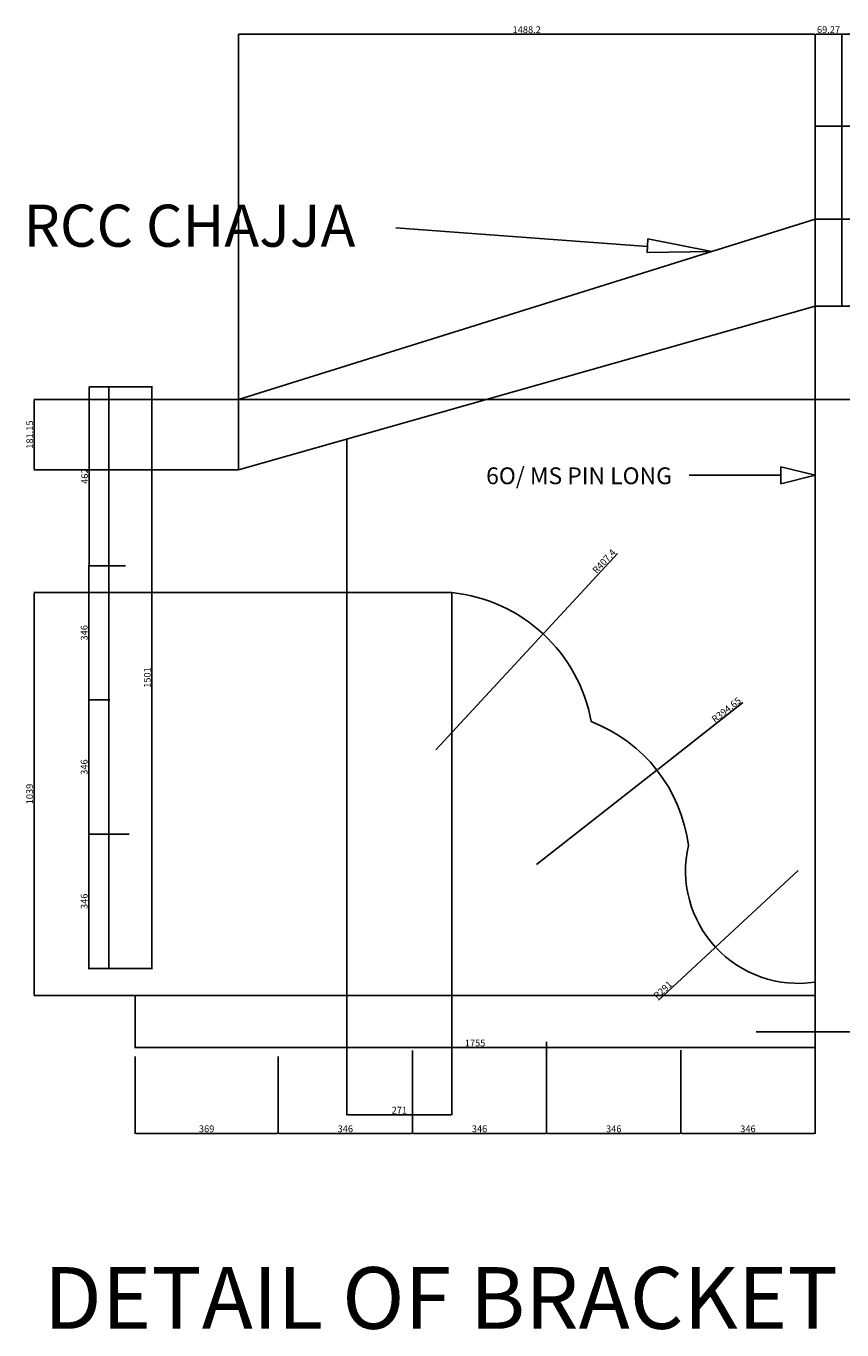
# Model space of a CAD drawing. Units: millimetres. Extents: x 498 to 8860, y -426 to 8717.
# Tile 3 of 9: x 5212 to 7317, y -15 to 3349. Entities that reach past the tile are written whole.
import ezdxf

# ---------------------------------------------------------------- set-up
doc = ezdxf.new("R2010")
doc.units = ezdxf.units.MM
for name, color, linetype, lineweight in [('A-ANNO-DIMS', 2, 'Continuous', 18), ('A-ANNO-TEXT', 3, 'Continuous', 18), ('A-DETL', 7, 'Continuous', 25)]:
    doc.layers.add(name, color=color, linetype=linetype, lineweight=lineweight)
doc.styles.get("Standard").update_dxf_attribs({"font": 'arial.ttf'})
doc.dimstyles.new('ISO-25', dxfattribs={"dimtxt": 17.5, "dimasz": 2.5, "dimexe": 1.25, "dimexo": 0.625, "dimtad": 1, "dimdec": 0, "dimtxsty": 'Standard', "dimcen": 2.5, "dimadec": 0, "dimazin": 0, "dimtfac": 1, "dimtdec": 0, "dimtmove": 0, "dimatfit": 3, "dimfxl": 1, "dimarcsym": 0})

# ---------------------------------------------------------------- blocks, each defined once
blk = doc.blocks.new('*D18')
at = {"layer": 'A-ANNO-DIMS', "color": 0, "lineweight": -2, "transparency": 16777216}
for p, q in [((5492.9, 690.8), (5492.9, 491.1)), ((5862.3, 690.9), (5862.3, 491.1)), ((5495.4, 492.3), (5859.8, 492.3))]:
    blk.add_line(p, q, dxfattribs=at)
at = {"layer": 'A-ANNO-DIMS', "color": 0, "transparency": 16777216}
for points in [[(5495.4, 492.8), (5495.4, 491.9), (5492.9, 492.3)], [(5859.8, 492.8), (5859.8, 491.9), (5862.3, 492.3)]]:
    blk.add_solid(points, dxfattribs=at)
at = {"layer": 'Defpoints', "color": 0, "transparency": 16777216}
for p in [(5492.9, 691.4), (5862.3, 691.5), (5862.3, 492.3)]:
    blk.add_point(p, dxfattribs=at)
at = {"layer": 'A-ANNO-DIMS', "color": 0, "transparency": 16777216, "insert": (5677.6, 501.9), "char_height": 17.5, "attachment_point": 5}
blk.add_mtext('369', dxfattribs=at)
blk = doc.blocks.new('*D19')
at = {"layer": 'A-ANNO-DIMS', "color": 0, "lineweight": -2, "transparency": 16777216}
for p, q in [((5862.3, 690.9), (5862.3, 491.1)), ((6208.7, 706.2), (6208.7, 491.1)), ((5864.8, 492.3), (6206.2, 492.3))]:
    blk.add_line(p, q, dxfattribs=at)
at = {"layer": 'A-ANNO-DIMS', "color": 0, "transparency": 16777216}
for points in [[(5864.8, 492.8), (5864.8, 491.9), (5862.3, 492.3)], [(6206.2, 492.8), (6206.2, 491.9), (6208.7, 492.3)]]:
    blk.add_solid(points, dxfattribs=at)
at = {"layer": 'Defpoints', "color": 0, "transparency": 16777216}
for p in [(6208.7, 706.9), (5862.3, 691.5), (6208.7, 492.3)]:
    blk.add_point(p, dxfattribs=at)
at = {"layer": 'A-ANNO-DIMS', "color": 0, "transparency": 16777216, "insert": (6035.5, 501.9), "char_height": 17.5, "attachment_point": 5}
blk.add_mtext('346', dxfattribs=at)
blk = doc.blocks.new('*D20')
at = {"layer": 'A-ANNO-DIMS', "color": 0, "lineweight": -2, "transparency": 16777216}
for p, q in [((6555, 728.6), (6555, 491.1)), ((6208.7, 706.2), (6208.7, 491.1)), ((6211.2, 492.3), (6552.5, 492.3))]:
    blk.add_line(p, q, dxfattribs=at)
at = {"layer": 'A-ANNO-DIMS', "color": 0, "transparency": 16777216}
for points in [[(6211.2, 492.8), (6211.2, 491.9), (6208.7, 492.3)], [(6552.5, 492.8), (6552.5, 491.9), (6555, 492.3)]]:
    blk.add_solid(points, dxfattribs=at)
at = {"layer": 'Defpoints', "color": 0, "transparency": 16777216}
for p in [(6208.7, 706.9), (6555, 729.2), (6555, 492.3)]:
    blk.add_point(p, dxfattribs=at)
at = {"layer": 'A-ANNO-DIMS', "color": 0, "transparency": 16777216, "insert": (6381.9, 501.9), "char_height": 17.5, "attachment_point": 5}
blk.add_mtext('346', dxfattribs=at)
blk = doc.blocks.new('*D21')
at = {"layer": 'A-ANNO-DIMS', "color": 0, "lineweight": -2, "transparency": 16777216}
for p, q in [((6901.4, 707.1), (6901.4, 491.1)), ((6555, 706.2), (6555, 491.1)), ((6557.5, 492.3), (6898.9, 492.3))]:
    blk.add_line(p, q, dxfattribs=at)
at = {"layer": 'A-ANNO-DIMS', "color": 0, "transparency": 16777216}
for points in [[(6557.5, 492.8), (6557.5, 491.9), (6555, 492.3)], [(6898.9, 492.8), (6898.9, 491.9), (6901.4, 492.3)]]:
    blk.add_solid(points, dxfattribs=at)
at = {"layer": 'Defpoints', "color": 0, "transparency": 16777216}
for p in [(6555, 706.9), (6901.4, 707.7), (6901.4, 492.3)]:
    blk.add_point(p, dxfattribs=at)
at = {"layer": 'A-ANNO-DIMS', "color": 0, "transparency": 16777216, "insert": (6728.2, 501.9), "char_height": 17.5, "attachment_point": 5}
blk.add_mtext('346', dxfattribs=at)
blk = doc.blocks.new('*D22')
at = {"layer": 'A-ANNO-DIMS', "color": 0, "lineweight": -2, "transparency": 16777216}
for p, q in [((6901.4, 707.1), (6901.4, 491.1)), ((7247.7, 713), (7247.7, 491.1)), ((6903.9, 492.3), (7245.2, 492.3))]:
    blk.add_line(p, q, dxfattribs=at)
at = {"layer": 'A-ANNO-DIMS', "color": 0, "transparency": 16777216}
for points in [[(6903.9, 492.8), (6903.9, 491.9), (6901.4, 492.3)], [(7245.2, 492.8), (7245.2, 491.9), (7247.7, 492.3)]]:
    blk.add_solid(points, dxfattribs=at)
at = {"layer": 'Defpoints', "color": 0, "transparency": 16777216}
for p in [(6901.4, 707.7), (7247.7, 713.6), (7247.7, 492.3)]:
    blk.add_point(p, dxfattribs=at)
at = {"layer": 'A-ANNO-DIMS', "color": 0, "transparency": 16777216, "insert": (7074.5, 501.9), "char_height": 17.5, "attachment_point": 5}
blk.add_mtext('346', dxfattribs=at)
blk = doc.blocks.new('*D23')
at = {"layer": 'A-ANNO-DIMS', "color": 0, "lineweight": -2, "transparency": 16777216}
for p, q in [((5483.9, 2418.8), (5373.6, 2418.8)), ((5374.8, 2416.3), (5374.8, 1959.5)), ((5468.5, 1957), (5373.6, 1957))]:
    blk.add_line(p, q, dxfattribs=at)
at = {"layer": 'A-ANNO-DIMS', "color": 0, "transparency": 16777216}
for points in [[(5374.4, 2416.3), (5375.2, 2416.3), (5374.8, 2418.8)], [(5374.4, 1959.5), (5375.2, 1959.5), (5374.8, 1957)]]:
    blk.add_solid(points, dxfattribs=at)
at = {"layer": 'Defpoints', "color": 0, "transparency": 16777216}
for p in [(5484.5, 2418.8), (5374.8, 1957), (5469.1, 1957)]:
    blk.add_point(p, dxfattribs=at)
at = {"layer": 'A-ANNO-DIMS', "color": 0, "transparency": 16777216, "insert": (5365.3, 2187.9), "char_height": 17.5, "attachment_point": 5, "rotation": 90}
blk.add_mtext('462', dxfattribs=at)
blk = doc.blocks.new('*D24')
at = {"layer": 'A-ANNO-DIMS', "color": 0, "lineweight": -2, "transparency": 16777216}
for p, q in [((5468.5, 1957), (5372.2, 1957)), ((5373.4, 1954.5), (5373.4, 1613.2)), ((5427.6, 1610.7), (5372.2, 1610.7))]:
    blk.add_line(p, q, dxfattribs=at)
at = {"layer": 'A-ANNO-DIMS', "color": 0, "transparency": 16777216}
for points in [[(5373, 1954.5), (5373.8, 1954.5), (5373.4, 1957)], [(5373, 1613.2), (5373.8, 1613.2), (5373.4, 1610.7)]]:
    blk.add_solid(points, dxfattribs=at)
at = {"layer": 'Defpoints', "color": 0, "transparency": 16777216}
for p in [(5469.1, 1957), (5373.4, 1610.7), (5428.2, 1610.7)]:
    blk.add_point(p, dxfattribs=at)
at = {"layer": 'A-ANNO-DIMS', "color": 0, "transparency": 16777216, "insert": (5363.9, 1783.9), "char_height": 17.5, "attachment_point": 5, "rotation": 90}
blk.add_mtext('346', dxfattribs=at)
blk = doc.blocks.new('*D25')
at = {"layer": 'A-ANNO-DIMS', "color": 0, "lineweight": -2, "transparency": 16777216}
for p, q in [((5427.6, 1610.7), (5372.2, 1610.7)), ((5373.4, 1608.2), (5373.4, 1266.8)), ((5477.9, 1264.3), (5372.2, 1264.3))]:
    blk.add_line(p, q, dxfattribs=at)
at = {"layer": 'A-ANNO-DIMS', "color": 0, "transparency": 16777216}
for points in [[(5373, 1608.2), (5373.8, 1608.2), (5373.4, 1610.7)], [(5373, 1266.8), (5373.8, 1266.8), (5373.4, 1264.3)]]:
    blk.add_solid(points, dxfattribs=at)
at = {"layer": 'Defpoints', "color": 0, "transparency": 16777216}
for p in [(5428.2, 1610.7), (5373.4, 1264.3), (5478.6, 1264.3)]:
    blk.add_point(p, dxfattribs=at)
at = {"layer": 'A-ANNO-DIMS', "color": 0, "transparency": 16777216, "insert": (5363.9, 1437.5), "char_height": 17.5, "attachment_point": 5, "rotation": 90}
blk.add_mtext('346', dxfattribs=at)
blk = doc.blocks.new('*D26')
at = {"layer": 'A-ANNO-DIMS', "color": 0, "lineweight": -2, "transparency": 16777216}
for p, q in [((5477.9, 1264.3), (5372.2, 1264.3)), ((5373.4, 1261.8), (5373.4, 920.5)), ((5454.1, 918), (5372.2, 918))]:
    blk.add_line(p, q, dxfattribs=at)
at = {"layer": 'A-ANNO-DIMS', "color": 0, "transparency": 16777216}
for points in [[(5373, 1261.8), (5373.8, 1261.8), (5373.4, 1264.3)], [(5373, 920.5), (5373.8, 920.5), (5373.4, 918)]]:
    blk.add_solid(points, dxfattribs=at)
at = {"layer": 'Defpoints', "color": 0, "transparency": 16777216}
for p in [(5478.6, 1264.3), (5373.4, 918), (5454.7, 918)]:
    blk.add_point(p, dxfattribs=at)
at = {"layer": 'A-ANNO-DIMS', "color": 0, "transparency": 16777216, "insert": (5363.9, 1091.2), "char_height": 17.5, "attachment_point": 5, "rotation": 90}
blk.add_mtext('346', dxfattribs=at)
blk = doc.blocks.new('*D27')
at = {"layer": 'A-ANNO-DIMS', "color": 0, "lineweight": -2, "transparency": 16777216}
for p, q in [((5492.9, 847.8), (5492.9, 712.4)), ((7247.7, 847.8), (7247.7, 712.4)), ((5495.4, 713.6), (7245.2, 713.6))]:
    blk.add_line(p, q, dxfattribs=at)
at = {"layer": 'A-ANNO-DIMS', "color": 0, "transparency": 16777216}
for points in [[(5495.4, 714), (5495.4, 713.2), (5492.9, 713.6)], [(7245.2, 714), (7245.2, 713.2), (7247.7, 713.6)]]:
    blk.add_solid(points, dxfattribs=at)
at = {"layer": 'Defpoints', "color": 0, "transparency": 16777216}
for p in [(5492.9, 848.4), (7247.7, 848.4), (7247.7, 713.6)]:
    blk.add_point(p, dxfattribs=at)
at = {"layer": 'A-ANNO-DIMS', "color": 0, "transparency": 16777216, "insert": (6370.3, 723.2), "char_height": 17.5, "attachment_point": 5}
blk.add_mtext('1755', dxfattribs=at)
blk = doc.blocks.new('*D28')
at = {"layer": 'A-ANNO-DIMS', "color": 0, "lineweight": -2, "transparency": 16777216}
for p, q in [((5425.9, 2418.8), (5537.8, 2418.8)), ((5536.5, 920.5), (5536.5, 2416.3)), ((5410.3, 918), (5537.8, 918))]:
    blk.add_line(p, q, dxfattribs=at)
at = {"layer": 'A-ANNO-DIMS', "color": 0, "transparency": 16777216}
for points in [[(5536.1, 2416.3), (5536.9, 2416.3), (5536.5, 2418.8)], [(5536.1, 920.5), (5536.9, 920.5), (5536.5, 918)]]:
    blk.add_solid(points, dxfattribs=at)
at = {"layer": 'Defpoints', "color": 0, "transparency": 16777216}
for p in [(5425.3, 2418.8), (5536.5, 2418.8), (5409.7, 918)]:
    blk.add_point(p, dxfattribs=at)
at = {"layer": 'A-ANNO-DIMS', "color": 0, "transparency": 16777216, "insert": (5526.9, 1668.4), "char_height": 17.5, "attachment_point": 5, "rotation": 90}
blk.add_mtext('1501', dxfattribs=at)
blk = doc.blocks.new('*D66')
at = {"layer": 'A-ANNO-DIMS', "color": 0, "lineweight": -2, "transparency": 16777216}
for p, q in [((5758.9, 2385.7), (5231.5, 2385.7)), ((5232.7, 2383.2), (5232.7, 2207)), ((5758.9, 2204.5), (5231.5, 2204.5))]:
    blk.add_line(p, q, dxfattribs=at)
at = {"layer": 'A-ANNO-DIMS', "color": 0, "transparency": 16777216}
for points in [[(5232.3, 2383.2), (5233.1, 2383.2), (5232.7, 2385.7)], [(5232.3, 2207), (5233.1, 2207), (5232.7, 2204.5)]]:
    blk.add_solid(points, dxfattribs=at)
at = {"layer": 'Defpoints', "color": 0, "transparency": 16777216}
for p in [(5759.5, 2385.7), (5232.7, 2204.5), (5759.5, 2204.5)]:
    blk.add_point(p, dxfattribs=at)
at = {"layer": 'A-ANNO-DIMS', "color": 0, "transparency": 16777216, "insert": (5223.2, 2295.1), "char_height": 17.5, "attachment_point": 5, "rotation": 90}
blk.add_mtext('181.15', dxfattribs=at)
blk = doc.blocks.new('*D67')
at = {"layer": 'A-ANNO-DIMS', "color": 0, "lineweight": -2, "transparency": 16777216}
for p, q in [((5759.5, 2386.3), (5759.5, 3329.3)), ((5762, 3328.1), (7245.2, 3328.1)), ((7247.7, 2851.9), (7247.7, 3329.3))]:
    blk.add_line(p, q, dxfattribs=at)
at = {"layer": 'A-ANNO-DIMS', "color": 0, "transparency": 16777216}
for points in [[(5762, 3328.5), (5762, 3327.6), (5759.5, 3328.1)], [(7245.2, 3328.5), (7245.2, 3327.6), (7247.7, 3328.1)]]:
    blk.add_solid(points, dxfattribs=at)
at = {"layer": 'Defpoints', "color": 0, "transparency": 16777216}
for p in [(7247.7, 3328.1), (7247.7, 2851.2), (5759.5, 2385.7)]:
    blk.add_point(p, dxfattribs=at)
at = {"layer": 'A-ANNO-DIMS', "color": 0, "transparency": 16777216, "insert": (6503.6, 3337.6), "char_height": 17.5, "attachment_point": 5}
blk.add_mtext('1488.2', dxfattribs=at)
blk = doc.blocks.new('*D68')
at = {"layer": 'A-ANNO-DIMS', "color": 0, "lineweight": -2, "transparency": 16777216}
for p, q in [((7248.3, 2851.2), (8125.9, 2851.2)), ((8124.6, 2388.2), (8124.6, 2848.7)), ((5760.1, 2385.7), (8125.9, 2385.7))]:
    blk.add_line(p, q, dxfattribs=at)
at = {"layer": 'A-ANNO-DIMS', "color": 0, "transparency": 16777216}
for points in [[(8124.2, 2848.7), (8125, 2848.7), (8124.6, 2851.2)], [(8124.2, 2388.2), (8125, 2388.2), (8124.6, 2385.7)]]:
    blk.add_solid(points, dxfattribs=at)
at = {"layer": 'Defpoints', "color": 0, "transparency": 16777216}
for p in [(7247.7, 2851.2), (8124.6, 2851.2), (5759.5, 2385.7)]:
    blk.add_point(p, dxfattribs=at)
at = {"layer": 'A-ANNO-DIMS', "color": 0, "transparency": 16777216, "insert": (8115.1, 2618.5), "char_height": 17.5, "attachment_point": 5, "rotation": 90}
blk.add_mtext('465.5', dxfattribs=at)
blk = doc.blocks.new('*D69')
at = {"layer": 'A-ANNO-DIMS', "color": 0, "lineweight": -2, "transparency": 16777216}
for p, q in [((7247.7, 3091.6), (7247.7, 3329.3)), ((7250.2, 3328.1), (7683.9, 3328.1)), ((7686.4, 3091.6), (7686.4, 3329.3))]:
    blk.add_line(p, q, dxfattribs=at)
at = {"layer": 'A-ANNO-DIMS', "color": 0, "transparency": 16777216}
for points in [[(7250.2, 3328.5), (7250.2, 3327.6), (7247.7, 3328.1)], [(7683.9, 3328.5), (7683.9, 3327.6), (7686.4, 3328.1)]]:
    blk.add_solid(points, dxfattribs=at)
at = {"layer": 'Defpoints', "color": 0, "transparency": 16777216}
for p in [(7686.4, 3328.1), (7247.7, 3090.9), (7686.4, 3090.9)]:
    blk.add_point(p, dxfattribs=at)
at = {"layer": 'A-ANNO-DIMS', "color": 0, "transparency": 16777216, "insert": (7467.1, 3337.6), "char_height": 17.5, "attachment_point": 5}
blk.add_mtext('438.7', dxfattribs=at)
blk = doc.blocks.new('*D70')
at = {"layer": 'A-ANNO-DIMS', "color": 0, "lineweight": -2, "transparency": 16777216}
for p, q in [((7247.7, 2627.1), (7247.7, 3329.3)), ((7250.2, 3328.1), (7314.5, 3328.1)), ((7317, 2627.1), (7317, 3329.3))]:
    blk.add_line(p, q, dxfattribs=at)
at = {"layer": 'A-ANNO-DIMS', "color": 0, "transparency": 16777216}
for points in [[(7250.2, 3328.5), (7250.2, 3327.6), (7247.7, 3328.1)], [(7314.5, 3328.5), (7314.5, 3327.6), (7317, 3328.1)]]:
    blk.add_solid(points, dxfattribs=at)
at = {"layer": 'Defpoints', "color": 0, "transparency": 16777216}
for p in [(7317, 3328.1), (7247.7, 2626.5), (7317, 2626.5)]:
    blk.add_point(p, dxfattribs=at)
at = {"layer": 'A-ANNO-DIMS', "color": 0, "transparency": 16777216, "insert": (7282.4, 3337.6), "char_height": 17.5, "attachment_point": 5}
blk.add_mtext('69.27', dxfattribs=at)
blk = doc.blocks.new('*D72')
at = {"layer": 'A-ANNO-DIMS', "color": 0, "lineweight": -2, "transparency": 16777216}
for p, q in [((6038.8, 1887.4), (5231.5, 1887.4)), ((5232.7, 1884.9), (5232.7, 850.9)), ((5492.3, 848.4), (5231.5, 848.4))]:
    blk.add_line(p, q, dxfattribs=at)
at = {"layer": 'A-ANNO-DIMS', "color": 0, "transparency": 16777216}
for points in [[(5232.3, 1884.9), (5233.1, 1884.9), (5232.7, 1887.4)], [(5232.3, 850.9), (5233.1, 850.9), (5232.7, 848.4)]]:
    blk.add_solid(points, dxfattribs=at)
at = {"layer": 'Defpoints', "color": 0, "transparency": 16777216}
for p in [(6039.4, 1887.4), (5232.7, 848.4), (5492.9, 848.4)]:
    blk.add_point(p, dxfattribs=at)
at = {"layer": 'A-ANNO-DIMS', "color": 0, "transparency": 16777216, "insert": (5223.2, 1367.9), "char_height": 17.5, "attachment_point": 5, "rotation": 90}
blk.add_mtext('1039', dxfattribs=at)
blk = doc.blocks.new('*D73')
at = {"layer": 'A-ANNO-DIMS', "color": 0, "lineweight": -2, "transparency": 16777216}
for p, q in [((6039.4, 1886.8), (6039.4, 539.3)), ((6310.4, 1886.8), (6310.4, 539.3)), ((6041.9, 540.5), (6307.9, 540.5))]:
    blk.add_line(p, q, dxfattribs=at)
at = {"layer": 'A-ANNO-DIMS', "color": 0, "transparency": 16777216}
for points in [[(6041.9, 541), (6041.9, 540.1), (6039.4, 540.5)], [(6307.9, 541), (6307.9, 540.1), (6310.4, 540.5)]]:
    blk.add_solid(points, dxfattribs=at)
at = {"layer": 'Defpoints', "color": 0, "transparency": 16777216}
for p in [(6039.4, 1887.4), (6310.4, 1887.4), (6310.4, 540.5)]:
    blk.add_point(p, dxfattribs=at)
at = {"layer": 'A-ANNO-DIMS', "color": 0, "transparency": 16777216, "insert": (6174.9, 550), "char_height": 17.5, "attachment_point": 5}
blk.add_mtext('271', dxfattribs=at)
blk = doc.blocks.new('*D86')
at = {"layer": 'A-ANNO-DIMS', "color": 0, "lineweight": -2, "transparency": 16777216}
for p, q in [((6738, 1988.8), (6547.5, 1783)), ((6269.1, 1482.1), (6545.8, 1781.1))]:
    blk.add_line(p, q, dxfattribs=at)
at = {"layer": 'A-ANNO-DIMS', "color": 0, "transparency": 16777216}
blk.add_solid([(6547.2, 1783.2), (6547.8, 1782.7), (6545.8, 1781.1)], dxfattribs=at)
at = {"layer": 'Defpoints', "color": 0, "transparency": 16777216}
for p in [(6545.8, 1781.1), (6269.1, 1482.1)]:
    blk.add_point(p, dxfattribs=at)
at = {"layer": 'A-ANNO-DIMS', "color": 0, "transparency": 16777216, "insert": (6704.8, 1967), "char_height": 17.5, "attachment_point": 5, "rotation": 47.2169}
blk.add_mtext('R407.4', dxfattribs=at)
blk = doc.blocks.new('*D87')
at = {"layer": 'A-ANNO-DIMS', "color": 0, "lineweight": -2, "transparency": 16777216}
for p, q in [((7061.6, 1603.8), (6841.6, 1431.1)), ((6529.1, 1185.9), (6839.6, 1429.6))]:
    blk.add_line(p, q, dxfattribs=at)
at = {"layer": 'A-ANNO-DIMS', "color": 0, "transparency": 16777216}
blk.add_solid([(6841.3, 1431.5), (6841.8, 1430.8), (6839.6, 1429.6)], dxfattribs=at)
at = {"layer": 'Defpoints', "color": 0, "transparency": 16777216}
for p in [(6839.6, 1429.6), (6529.1, 1185.9)]:
    blk.add_point(p, dxfattribs=at)
at = {"layer": 'A-ANNO-DIMS', "color": 0, "transparency": 16777216, "insert": (7020, 1583.3), "char_height": 17.5, "attachment_point": 5, "rotation": 38.1232}
blk.add_mtext('R394.65', dxfattribs=at)
blk = doc.blocks.new('*D88')
at = {"layer": 'A-ANNO-DIMS', "color": 0, "lineweight": -2, "transparency": 16777216}
for p, q in [((7204.4, 1170.4), (6991, 972.5)), ((6843.5, 835.7), (6989.2, 970.8))]:
    blk.add_line(p, q, dxfattribs=at)
at = {"layer": 'A-ANNO-DIMS', "color": 0, "transparency": 16777216}
blk.add_solid([(6988.9, 971.1), (6989.5, 970.5), (6991, 972.5)], dxfattribs=at)
at = {"layer": 'Defpoints', "color": 0, "transparency": 16777216}
for p in [(7204.4, 1170.4), (6991, 972.5)]:
    blk.add_point(p, dxfattribs=at)
at = {"layer": 'A-ANNO-DIMS', "color": 0, "transparency": 16777216, "insert": (6856.5, 860.8), "char_height": 17.5, "attachment_point": 5, "rotation": 42.8468}
blk.add_mtext('R291', dxfattribs=at)

msp = doc.modelspace()

# ---------------------------------------------------------------- linework, layer by layer
at = {"layer": 'A-DETL'}
for p, q in [((7247.72, 2851.24), (7247.72, 3090.936)), ((5759.508, 2385.702), (7247.72, 2851.24)), ((6166.245, 2828.784), (6815.441, 2780.347)), ((6814.708, 2764.681), (6816.389, 2800.614)), ((6816.389, 2800.614), (6981.487, 2767.958)), ((6815.441, 2780.347), (6814.708, 2764.681)), ((6981.487, 2767.958), (6814.708, 2764.681)), ((7247.72, 2626.504), (5759.508, 2204.548)), ((7247.72, 754.555), (7247.72, 2626.504)), ((7247.72, 2626.504), (7686.422, 2626.504)), ((5425.229, 918.005), (5425.229, 2418.828)), ((5759.508, 2204.548), (5759.508, 2385.702)), ((6039.413, 1887.42), (6039.413, 2283.911)), ((6922.953, 2190.666), (7159.598, 2190.666)), ((7159.598, 2190.666), (7159.598, 2211.817)), ((7159.598, 2211.817), (7159.598, 2168.065)), ((7247.72, 2190.666), (7159.598, 2211.817)), ((7159.598, 2168.065), (7247.72, 2190.666)), ((5425.229, 1610.692), (5425.229, 1957.036)), ((6310.396, 1887.42), (6039.413, 1887.42)), ((5425.229, 1264.349), (5425.229, 1610.692)), ((5425.229, 918.005), (5425.229, 1264.349)), ((5492.912, 848.389), (7247.72, 848.389)), ((5492.912, 848.389), (5862.345, 848.389)), ((5862.345, 848.389), (6208.689, 848.389)), ((6208.689, 848.389), (6555.033, 848.389)), ((6555.033, 848.389), (6901.377, 848.389)), ((7247.72, 754.555), (7686.422, 754.555))]:
    msp.add_line(p, q, dxfattribs=at)
for points in [[(7247.72, 3090.936), (7434.589, 3090.936), (7450.83, 3046.314), (7483.312, 3135.559), (7499.554, 3090.936), (7686.422, 3090.936)], [(7095.919, 754.555), (7451.409, 754.555), (7459.24, 733.039), (7474.902, 776.07), (7482.733, 754.555), (7833.194, 754.555)]]:
    msp.add_lwpolyline(points, dxfattribs=at)
for centre, radius, start, end in [((6269.121, 1482.137), 407.379, 10.245175, 84.184984), ((6529.119, 1185.948), 394.65, 7.166624, 69.08453), ((7204.362, 1170.399), 290.98, 167.135886, 278.569491)]:
    msp.add_arc(centre, radius, start, end, dxfattribs=at)

# ---------------------------------------------------------------- texts
at = {"layer": 'A-ANNO-TEXT'}
for s, height, p in [('RCC CHAJJA', 108.4825, (5205.118, 2779.87)), ('6O/ MS PIN LONG', 43.2958, (6398.889, 2167.255)), ('DETAIL OF BRACKET', 159.20004, (5257.522, -11.793))]:
    msp.add_text(s, height=height, dxfattribs=at).set_placement(p)

# ---------------------------------------------------------------- dimensions: what is measured, and where the dimension line sits
at = {"layer": 'A-ANNO-DIMS'}
for base, p1, p2, override, picture, middle in [((7247.72, 3328.059), (5759.508, 2385.702), (7247.72, 2851.24), {"dimdec": 1, "dimlfac": 1, "dimrnd": 0, "dimzin": 0, "dimdsep": 46, "dimlunit": 2}, '*D67', (6503.614, 3337.619)), ((7686.422, 3328.059), (7247.72, 3090.936), (7686.422, 3090.936), {"dimdec": 1, "dimlfac": 1, "dimrnd": 0, "dimzin": 0, "dimdsep": 46, "dimlunit": 2}, '*D69', (7467.071, 3337.625)), ((7316.989, 3328.059), (7247.72, 2626.504), (7316.989, 2626.504), {"dimdec": 2, "dimlfac": 1, "dimrnd": 0, "dimzin": 0, "dimdsep": 46, "dimlunit": 2}, '*D70', (7282.355, 3337.619)), ((6310.396, 540.539), (6039.413, 1887.42), (6310.396, 1887.42), {"dimdec": 0, "dimlfac": 1, "dimrnd": 0, "dimzin": 0, "dimdsep": 46, "dimlunit": 2}, '*D73', (6174.904, 549.95)), ((7247.72, 713.619), (5492.912, 848.389), (7247.72, 848.389), {"dimclrd": 0, "dimclre": 0, "dimclrt": 0}, '*D27', (6370.316, 723.179)), ((6208.689, 492.34), (5862.345, 691.512), (6208.689, 706.857), {"dimclrd": 0, "dimclre": 0, "dimclrt": 0}, '*D19', (6035.517, 501.906)), ((6555.033, 492.34), (6208.689, 706.857), (6555.033, 729.196), {"dimclrd": 0, "dimclre": 0, "dimclrt": 0}, '*D20', (6381.861, 501.906)), ((6901.377, 492.34), (6555.033, 706.857), (6901.377, 707.74), {"dimclrd": 0, "dimclre": 0, "dimclrt": 0}, '*D21', (6728.205, 501.906)), ((7247.72, 492.34), (6901.377, 707.74), (7247.72, 713.619), {"dimclrd": 0, "dimclre": 0, "dimclrt": 0}, '*D22', (7074.548, 501.906)), ((5862.345, 492.34), (5492.912, 691.416), (5862.345, 691.512), {"dimclrd": 0, "dimclre": 0, "dimclrt": 0}, '*D18', (5677.629, 501.906))]:
    dim = msp.add_linear_dim(base=base, p1=p1, p2=p2, dimstyle='ISO-25', override=override, dxfattribs=at)
    dim.commit()
    dim.dimension.update_dxf_attribs({"geometry": picture, "text_midpoint": middle})
for base, p1, p2, override, picture, middle in [((8124.627, 2851.24), (5759.508, 2385.702), (7247.72, 2851.24), {"dimdec": 1, "dimlfac": 1, "dimrnd": 0, "dimzin": 0, "dimdsep": 46, "dimlunit": 2}, '*D68', (8115.067, 2618.471)), ((5374.831, 1957.036), (5484.476, 2418.828), (5469.136, 1957.036), {"dimclrd": 0, "dimclre": 0, "dimclrt": 0}, '*D23', (5365.271, 2187.932)), ((5536.505, 2418.828), (5409.724, 918.005), (5425.324, 2418.828), {"dimclrd": 0, "dimclre": 0, "dimclrt": 0}, '*D28', (5526.945, 1668.416)), ((5232.729, 2204.548), (5759.508, 2385.702), (5759.508, 2204.548), {"dimdec": 2, "dimlfac": 1, "dimrnd": 0, "dimzin": 0, "dimdsep": 46, "dimlunit": 2}, '*D66', (5223.169, 2295.125)), ((5373.428, 1610.692), (5469.136, 1957.036), (5428.186, 1610.692), {"dimclrd": 0, "dimclre": 0, "dimclrt": 0}, '*D24', (5363.862, 1783.864)), ((5232.729, 848.389), (6039.413, 1887.42), (5492.912, 848.389), {"dimdec": 0, "dimlfac": 1, "dimrnd": 0, "dimzin": 0, "dimdsep": 46, "dimlunit": 2}, '*D72', (5223.163, 1367.904)), ((5373.428, 1264.349), (5428.186, 1610.692), (5478.568, 1264.349), {"dimclrd": 0, "dimclre": 0, "dimclrt": 0}, '*D25', (5363.862, 1437.521)), ((5373.428, 918.005), (5478.568, 1264.349), (5454.678, 918.005), {"dimclrd": 0, "dimclre": 0, "dimclrt": 0}, '*D26', (5363.862, 1091.177))]:
    dim = msp.add_linear_dim(base=base, p1=p1, p2=p2, angle=90, dimstyle='ISO-25', override=override, dxfattribs=at)
    dim.commit()
    dim.dimension.update_dxf_attribs({"geometry": picture, "text_midpoint": middle})
for center, mpoint, override, picture, middle in [((6269.121, 1482.137), (6545.823, 1781.125), {"dimdec": 1, "dimlfac": 1, "dimrnd": 0, "dimzin": 0, "dimdsep": 46, "dimlunit": 2}, '*D86', (6711.844, 1960.517)), ((6529.119, 1185.948), (6839.584, 1429.587), {"dimdec": 2, "dimlfac": 1, "dimrnd": 0, "dimzin": 0, "dimdsep": 46, "dimlunit": 2}, '*D87', (7025.863, 1575.771)), ((7204.362, 1170.399), (6991.023, 972.521), {"dimdec": 0, "dimlfac": 1, "dimrnd": 0, "dimzin": 0, "dimdsep": 46, "dimlunit": 2}, '*D88', (6863.019, 853.794))]:
    dim = msp.add_radius_dim(center=center, mpoint=mpoint, dimstyle='ISO-25', override=override, dxfattribs=at)
    dim.commit()
    dim.dimension.update_dxf_attribs({"geometry": picture, "text_midpoint": middle, "dimtype": 164})

doc.saveas('drawing.dxf')
